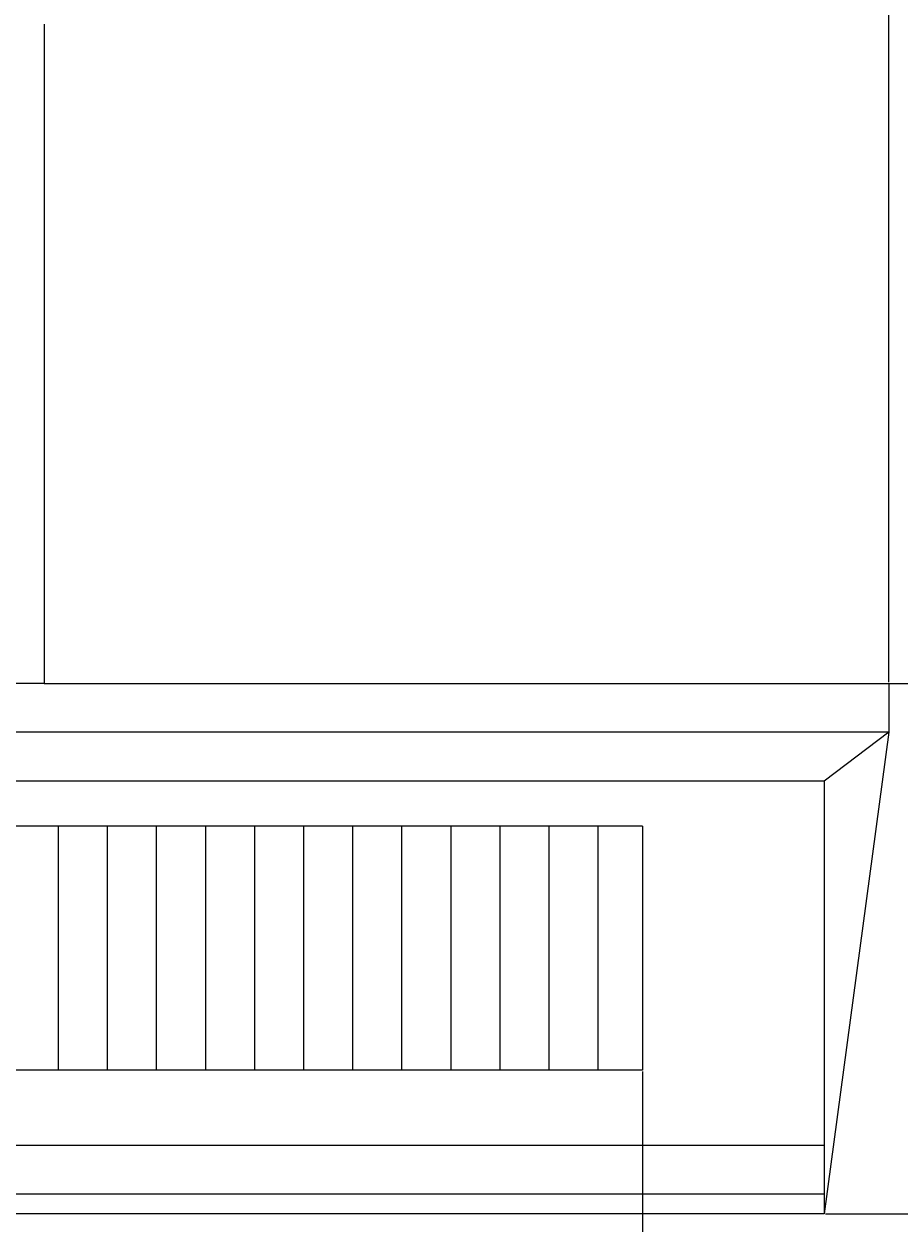
# Model space of a CAD drawing. Units: millimetres. Extents: x 2332 to 5836, y -853 to 2199.
# Tile 11 of 16: x 4331 to 4779, y 753 to 1368. Entities that reach past the tile are written whole.
import ezdxf

# ---------------------------------------------------------------- set-up
doc = ezdxf.new("R2010")
doc.units = ezdxf.units.MM
for name, color, linetype, lineweight in [('A-ANNO-DIMS', 2, 'Continuous', 18), ('A-EQPM', 7, 'Continuous', 25), ('A-EQPM-PATT', 7, 'Continuous', 13)]:
    doc.layers.add(name, color=color, linetype=linetype, lineweight=lineweight)
doc.styles.get("Standard").update_dxf_attribs({"font": 'arial.ttf'})
doc.dimstyles.new('ISO-25', dxfattribs={"dimtxt": 2.5, "dimasz": 2.5, "dimexe": 1.25, "dimexo": 0.625, "dimtad": 1, "dimtxsty": 'Standard', "dimcen": 2.5, "dimadec": 0, "dimazin": 0, "dimtfac": 1, "dimtmove": 0, "dimatfit": 3, "dimfxl": 1, "dimarcsym": 0})

# ---------------------------------------------------------------- blocks, each defined once
blk = doc.blocks.new('*D23')
at = {"layer": 'A-ANNO-DIMS', "color": 0, "lineweight": -2, "transparency": 16777216}
for p, q in [((3646.47, 1030.43), (3646.47, 2168.7)), ((3648.97, 2167.45), (4771.11, 2167.45)), ((4773.61, 1030.43), (4773.61, 2168.7))]:
    blk.add_line(p, q, dxfattribs=at)
at = {"layer": 'A-ANNO-DIMS', "color": 0, "transparency": 16777216}
for points in [[(3648.97, 2167.87), (3648.97, 2167.04), (3646.47, 2167.45)], [(4771.11, 2167.87), (4771.11, 2167.04), (4773.61, 2167.45)]]:
    blk.add_solid(points, dxfattribs=at)
at = {"layer": 'Defpoints', "color": 0, "transparency": 16777216}
for p in [(4773.61, 2167.45), (3646.47, 1029.8), (4773.61, 1029.8)]:
    blk.add_point(p, dxfattribs=at)
at = {"layer": 'A-ANNO-DIMS', "color": 0, "transparency": 16777216, "insert": (4210.04, 2169.33), "char_height": 2.5, "attachment_point": 5}
blk.add_mtext('1127.1', dxfattribs=at)
blk = doc.blocks.new('*D25')
at = {"layer": 'A-ANNO-DIMS', "color": 0, "lineweight": -2, "transparency": 16777216}
for p, q in [((4341.52, 1705.81), (5835.94, 1705.81)), ((5834.69, 1032.3), (5834.69, 1703.31)), ((4341.52, 1029.8), (5835.94, 1029.8))]:
    blk.add_line(p, q, dxfattribs=at)
at = {"layer": 'A-ANNO-DIMS', "color": 0, "transparency": 16777216}
for points in [[(5834.27, 1703.31), (5835.11, 1703.31), (5834.69, 1705.81)], [(5834.27, 1032.3), (5835.11, 1032.3), (5834.69, 1029.8)]]:
    blk.add_solid(points, dxfattribs=at)
at = {"layer": 'Defpoints', "color": 0, "transparency": 16777216}
for p in [(4340.89, 1705.81), (5834.69, 1705.81), (4340.89, 1029.8)]:
    blk.add_point(p, dxfattribs=at)
at = {"layer": 'A-ANNO-DIMS', "color": 0, "transparency": 16777216, "insert": (5832.79, 1367.8), "char_height": 2.5, "attachment_point": 5, "rotation": 90}
blk.add_mtext('676', dxfattribs=at)
blk = doc.blocks.new('*D26')
at = {"layer": 'A-ANNO-DIMS', "color": 0, "lineweight": -2, "transparency": 16777216}
for p, q in [((4774.24, 1029.8), (5835.94, 1029.8)), ((5834.69, 760.56), (5834.69, 1027.3)), ((4741.16, 758.06), (5835.94, 758.06))]:
    blk.add_line(p, q, dxfattribs=at)
at = {"layer": 'A-ANNO-DIMS', "color": 0, "transparency": 16777216}
for points in [[(5834.27, 1027.3), (5835.11, 1027.3), (5834.69, 1029.8)], [(5834.27, 760.56), (5835.11, 760.56), (5834.69, 758.06)]]:
    blk.add_solid(points, dxfattribs=at)
at = {"layer": 'Defpoints', "color": 0, "transparency": 16777216}
for p in [(4773.61, 1029.8), (5834.69, 1029.8), (4740.54, 758.06)]:
    blk.add_point(p, dxfattribs=at)
at = {"layer": 'A-ANNO-DIMS', "color": 0, "transparency": 16777216, "insert": (5832.81, 893.93), "char_height": 2.5, "attachment_point": 5, "rotation": 90}
blk.add_mtext('271.74', dxfattribs=at)
blk = doc.blocks.new('*D27')
at = {"layer": 'A-ANNO-DIMS', "color": 0, "lineweight": -2, "transparency": 16777216}
for p, q in [((3772.66, 830.99), (3772.66, -853.1)), ((4647.42, 830.99), (4647.42, -853.1)), ((3775.16, -851.85), (4644.92, -851.85))]:
    blk.add_line(p, q, dxfattribs=at)
at = {"layer": 'A-ANNO-DIMS', "color": 0, "transparency": 16777216}
for points in [[(3775.16, -851.43), (3775.16, -852.26), (3772.66, -851.85)], [(4644.92, -851.43), (4644.92, -852.26), (4647.42, -851.85)]]:
    blk.add_solid(points, dxfattribs=at)
at = {"layer": 'Defpoints', "color": 0, "transparency": 16777216}
for p in [(3772.66, 831.62), (4647.42, 831.62), (4647.42, -851.85)]:
    blk.add_point(p, dxfattribs=at)
at = {"layer": 'A-ANNO-DIMS', "color": 0, "transparency": 16777216, "insert": (4210.04, -849.95), "char_height": 2.5, "attachment_point": 5}
blk.add_mtext('874.8', dxfattribs=at)

msp = doc.modelspace()

# ---------------------------------------------------------------- hatches: boundary and pattern name
at = {"layer": 'A-EQPM-PATT'}
h = msp.add_hatch(dxfattribs=at)
h.set_pattern_fill('ANSI31', color=256, scale=7.9164, angle=45, style=0)
h.paths.add_polyline_path([(3772.661, 831.62), (4647.419, 831.62), (4647.419, 956.62), (3772.661, 956.62)])

# ---------------------------------------------------------------- linework, layer by layer
at = {"layer": 'A-EQPM'}
for p, q in [((4340.894, 1367.803), (4340.894, 1029.801)), ((4340.894, 1029.801), (4210.04, 1029.801)), ((4340.894, 1029.801), (4773.612, 1029.801)), ((4773.612, 1029.801), (4773.612, 1004.801)), ((4773.612, 1004.801), (4210.04, 1004.801)), ((4773.612, 1004.801), (4740.539, 979.768)), ((4773.612, 1004.801), (4740.539, 758.058)), ((4740.539, 979.768), (4210.04, 979.768)), ((4740.539, 979.768), (4740.539, 758.058)), ((4647.419, 956.62), (4210.04, 956.62)), ((4647.419, 956.62), (4647.419, 831.62)), ((4647.419, 831.62), (4210.04, 831.62)), ((4740.539, 793.058), (4210.04, 793.058)), ((4740.539, 768.058), (4210.04, 768.058)), ((4740.539, 758.058), (4210.04, 758.058))]:
    msp.add_line(p, q, dxfattribs=at)

# ---------------------------------------------------------------- dimensions: what is measured, and where the dimension line sits
at = {"layer": 'A-ANNO-DIMS'}
for base, p1, p2, picture, middle in [((4773.612, 2167.453), (3646.468, 1029.801), (4773.612, 1029.801), '*D23', (4210.04, 2169.334)), ((4647.419, -851.847), (3772.661, 831.62), (4647.419, 831.62), '*D27', (4210.04, -849.945))]:
    dim = msp.add_linear_dim(base=base, p1=p1, p2=p2, dimstyle='ISO-25', override={"dimdec": 1, "dimlfac": 1, "dimrnd": 0, "dimzin": 0, "dimdsep": 46, "dimlunit": 2}, dxfattribs=at)
    dim.commit()
    dim.dimension.update_dxf_attribs({"geometry": picture, "text_midpoint": middle})
for base, p1, p2, override, picture, middle in [((5834.69, 1705.805), (4340.894, 1029.801), (4340.894, 1705.805), {"dimdec": 0, "dimlfac": 1, "dimrnd": 0, "dimzin": 0, "dimdsep": 46, "dimlunit": 2}, '*D25', (5832.788, 1367.803)), ((5834.69, 1029.801), (4740.539, 758.058), (4773.612, 1029.801), {"dimdec": 2, "dimlfac": 1, "dimrnd": 0, "dimzin": 0, "dimdsep": 46, "dimlunit": 2}, '*D26', (5832.81, 893.93))]:
    dim = msp.add_linear_dim(base=base, p1=p1, p2=p2, angle=90, dimstyle='ISO-25', override=override, dxfattribs=at)
    dim.commit()
    dim.dimension.update_dxf_attribs({"geometry": picture, "text_midpoint": middle})

doc.saveas('drawing.dxf')
